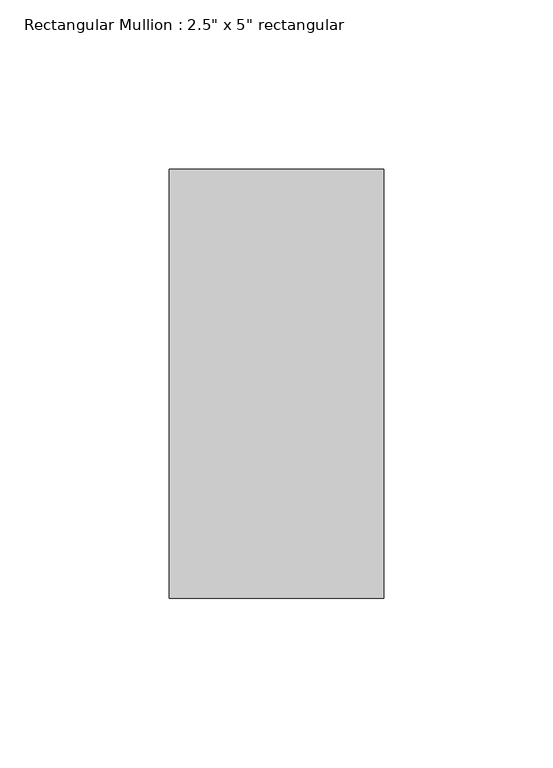
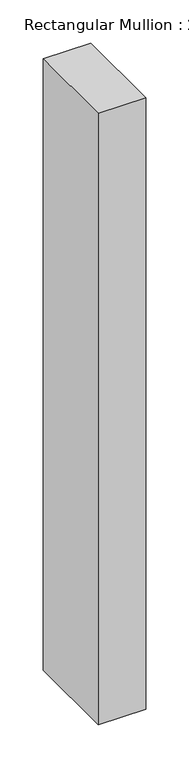
"""IFC4 building model written with IfcOpenShell, lengths in millimetres: member geometry."""

from ifc_helpers import new_model, si_unit, frame, origin, place, context, project, spatial, polyline, outline, extrude, source, transform, mapped, element, save


def member_b70ee1cc(model_context):
    return source(origin(), model_context, "Body", "SweptSolid", [
        extrude(outline(polyline([(0.0, 63.5), (0.0, -63.5), (-63.5, -63.5), (-63.5, 63.5), (0.0, 63.5)])), frame((0.0, 0.0, -863.6), z_axis=(0.0, 0.0, 1.0), x_axis=(1.0, 0.0, 0.0)), (0.0, 0.0, 1.0), 863.6),
    ])


if __name__ == "__main__":
    model = new_model("IFC4")
    model_context = context("Model", 3, world=origin())
    ifc_project = project(units=[si_unit("LENGTHUNIT", "METRE", prefix="MILLI")], contexts=[model_context])
    site = spatial("IfcSite", under=ifc_project)
    building = spatial("IfcBuilding", under=site)
    placement = place(None, origin())
    member_shape = member_b70ee1cc(model_context)
    element("IfcMember", 1, ObjectType="Rectangular Mullion : 2.5\" x 5\" rectangular", at=placement, inside=building, context=model_context, shape_type="MappedRepresentation", body=[
        mapped(member_shape, transform((0.0, 0.0, 0.0), x_axis=(1.0, 0.0, 0.0), y_axis=(0.0, 1.0, 0.0), z_axis=(0.0, 0.0, 1.0))),
    ])
    save(model, "model.ifc")

# Revit data of these elements
# Type "Rectangular Mullion : 2.5\" x 5\" rectangular"
#   built-in parameter 1007304 = 0.416667 (stored number, unit not read)
#   built-in parameter 1007301 = 0.104167 (stored number, unit not read)
#   built-in parameter 1007300 = 0.104167 (stored number, unit not read)
# Element 1 (IfcMember, "Rectangular Mullion : 2.5\" x 5\" rectangular")
#   Materials on its faces: "door colour"
# Materials
#   "door colour": class "Generic", colour RGB 120 120 120, transparency 0, Cost = 0
